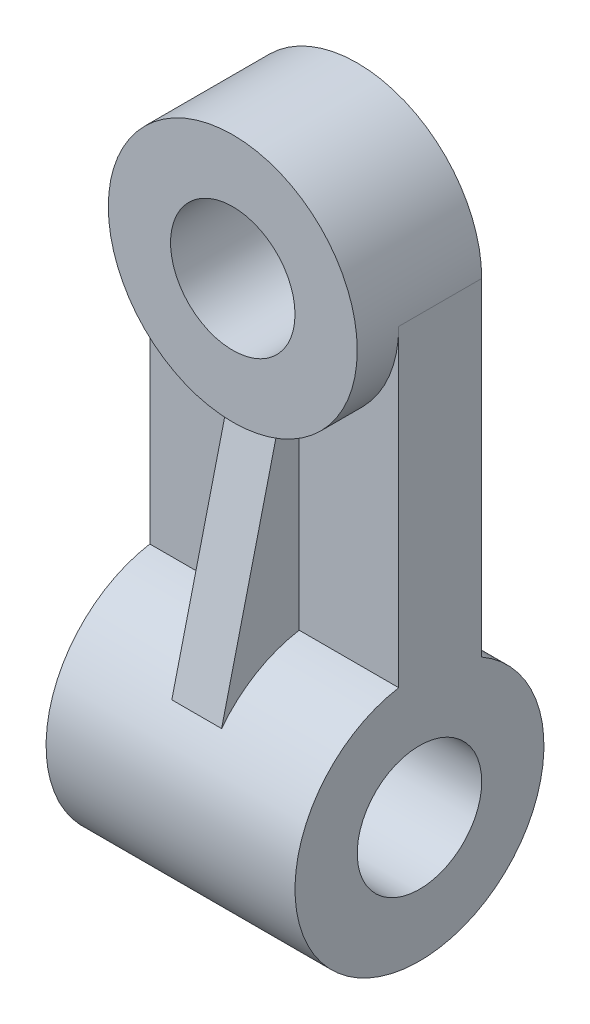
ISO-10303-21;
HEADER;
FILE_DESCRIPTION(('STEP AP214'),'2;1');
FILE_NAME('part.step','',(''),(''),'','','');
FILE_SCHEMA(('AUTOMOTIVE_DESIGN { 1 0 10303 214 1 1 1 1 }'));
ENDSEC;
DATA;
#1=APPLICATION_CONTEXT('core data for automotive mechanical design processes');
#2=APPLICATION_PROTOCOL_DEFINITION('international standard','automotive_design',2000,#1);
#3=PRODUCT_CONTEXT('',#1,'mechanical');
#4=PRODUCT('Part','Part','',(#3));
#5=PRODUCT_RELATED_PRODUCT_CATEGORY('part','',(#4));
#6=PRODUCT_DEFINITION_FORMATION('','',#4);
#7=PRODUCT_DEFINITION_CONTEXT('part definition',#1,'design');
#8=PRODUCT_DEFINITION('design','',#6,#7);
#9=PRODUCT_DEFINITION_SHAPE('','',#8);
#10=(LENGTH_UNIT() NAMED_UNIT(*) SI_UNIT(.MILLI.,.METRE.));
#11=(NAMED_UNIT(*) PLANE_ANGLE_UNIT() SI_UNIT($,.RADIAN.));
#12=(NAMED_UNIT(*) SI_UNIT($,.STERADIAN.) SOLID_ANGLE_UNIT());
#13=UNCERTAINTY_MEASURE_WITH_UNIT(LENGTH_MEASURE(1.E-05),#10,'distance_accuracy_value','');
#14=(GEOMETRIC_REPRESENTATION_CONTEXT(3) GLOBAL_UNCERTAINTY_ASSIGNED_CONTEXT((#13)) GLOBAL_UNIT_ASSIGNED_CONTEXT((#10,
#11,#12)) REPRESENTATION_CONTEXT('',''));
#15=CARTESIAN_POINT('',(0.,0.,0.));
#16=DIRECTION('',(0.,0.,1.));
#17=DIRECTION('',(1.,0.,0.));
#18=AXIS2_PLACEMENT_3D('',#15,#16,#17);
#19=CARTESIAN_POINT('',(30.,0.,20.));
#20=DIRECTION('',(0.,0.,-1.));
#21=DIRECTION('',(-1.,0.,0.));
#22=AXIS2_PLACEMENT_3D('',#19,#20,#21);
#23=PLANE('',#22);
#24=DIRECTION('',(0.,-1.,0.));
#25=VECTOR('',#24,1.);
#26=CARTESIAN_POINT('',(-6.,0.,20.));
#27=LINE('',#26,#25);
#28=CARTESIAN_POINT('',(-6.,-29.3938769133981,20.));
#29=VERTEX_POINT('',#28);
#30=CARTESIAN_POINT('',(-5.99999999999999,-75.4196010845019,20.));
#31=VERTEX_POINT('',#30);
#32=EDGE_CURVE('E116',#29,#31,#27,.T.);
#33=ORIENTED_EDGE('',*,*,#32,.F.);
#34=CARTESIAN_POINT('',(0.,0.,20.));
#35=DIRECTION('',(0.,0.,-1.));
#36=DIRECTION('',(-1.,0.,0.));
#37=AXIS2_PLACEMENT_3D('',#34,#35,#36);
#38=CIRCLE('',#37,30.);
#39=CARTESIAN_POINT('',(-30.,0.,20.));
#40=VERTEX_POINT('',#39);
#41=EDGE_CURVE('E160',#29,#40,#38,.T.);
#42=ORIENTED_EDGE('',*,*,#41,.T.);
#43=DIRECTION('',(0.,-1.,0.));
#44=VECTOR('',#43,1.);
#45=CARTESIAN_POINT('',(-30.,0.,20.));
#46=LINE('',#45,#44);
#47=CARTESIAN_POINT('',(-30.,-75.4196010845019,20.));
#48=VERTEX_POINT('',#47);
#49=EDGE_CURVE('E159',#40,#48,#46,.T.);
#50=ORIENTED_EDGE('',*,*,#49,.T.);
#51=DIRECTION('',(-1.,0.,0.));
#52=VECTOR('',#51,1.);
#53=CARTESIAN_POINT('',(30.,-75.4196010845019,20.));
#54=LINE('',#53,#52);
#55=EDGE_CURVE('E139',#31,#48,#54,.T.);
#56=ORIENTED_EDGE('',*,*,#55,.F.);
#57=EDGE_LOOP('',(#33,#42,#50,#56));
#58=FACE_BOUND('',#57,.T.);
#59=ADVANCED_FACE('F39',(#58),#23,.F.);
#60=CARTESIAN_POINT('',(0.,0.,0.));
#61=DIRECTION('',(0.,0.,1.));
#62=DIRECTION('',(1.,0.,0.));
#63=AXIS2_PLACEMENT_3D('',#60,#61,#62);
#64=PLANE('',#63);
#65=CARTESIAN_POINT('',(0.,0.,0.));
#66=DIRECTION('',(0.,0.,1.));
#67=DIRECTION('',(1.,0.,0.));
#68=AXIS2_PLACEMENT_3D('',#65,#66,#67);
#69=CIRCLE('',#68,15.);
#70=CARTESIAN_POINT('',(15.,0.,0.));
#71=VERTEX_POINT('',#70);
#72=EDGE_CURVE('E169',#71,#71,#69,.T.);
#73=ORIENTED_EDGE('',*,*,#72,.T.);
#74=EDGE_LOOP('',(#73));
#75=FACE_BOUND('',#74,.T.);
#76=DIRECTION('',(0.,1.,0.));
#77=VECTOR('',#76,1.);
#78=CARTESIAN_POINT('',(30.,-80.,0.));
#79=LINE('',#78,#77);
#80=CARTESIAN_POINT('',(30.,-79.0192378864668,0.));
#81=VERTEX_POINT('',#80);
#82=CARTESIAN_POINT('',(30.,0.,0.));
#83=VERTEX_POINT('',#82);
#84=EDGE_CURVE('E152',#81,#83,#79,.T.);
#85=ORIENTED_EDGE('',*,*,#84,.F.);
#86=DIRECTION('',(-1.,0.,0.));
#87=VECTOR('',#86,1.);
#88=CARTESIAN_POINT('',(30.,-79.0192378864668,0.));
#89=LINE('',#88,#87);
#90=CARTESIAN_POINT('',(-30.,-79.0192378864668,0.));
#91=VERTEX_POINT('',#90);
#92=EDGE_CURVE('E143',#91,#81,#89,.F.);
#93=ORIENTED_EDGE('',*,*,#92,.F.);
#94=DIRECTION('',(0.,1.,0.));
#95=VECTOR('',#94,1.);
#96=CARTESIAN_POINT('',(-30.,-80.,0.));
#97=LINE('',#96,#95);
#98=CARTESIAN_POINT('',(-30.,0.,0.));
#99=VERTEX_POINT('',#98);
#100=EDGE_CURVE('E151',#91,#99,#97,.T.);
#101=ORIENTED_EDGE('',*,*,#100,.T.);
#102=CARTESIAN_POINT('',(0.,0.,0.));
#103=DIRECTION('',(0.,0.,1.));
#104=DIRECTION('',(1.,0.,0.));
#105=AXIS2_PLACEMENT_3D('',#102,#103,#104);
#106=CIRCLE('',#105,30.);
#107=EDGE_CURVE('E175',#83,#99,#106,.T.);
#108=ORIENTED_EDGE('',*,*,#107,.F.);
#109=EDGE_LOOP('',(#85,#93,#101,#108));
#110=FACE_BOUND('',#109,.T.);
#111=ADVANCED_FACE('F183',(#75,#110),#64,.F.);
#112=CARTESIAN_POINT('',(30.,0.,20.));
#113=VERTEX_POINT('',#112);
#114=CARTESIAN_POINT('',(6.,-29.3938769133981,20.));
#115=VERTEX_POINT('',#114);
#116=EDGE_CURVE('E164',#113,#115,#38,.T.);
#117=ORIENTED_EDGE('',*,*,#116,.T.);
#118=DIRECTION('',(0.,-1.,0.));
#119=VECTOR('',#118,1.);
#120=CARTESIAN_POINT('',(6.,0.,20.));
#121=LINE('',#120,#119);
#122=CARTESIAN_POINT('',(6.00000000000001,-75.4196010845019,20.));
#123=VERTEX_POINT('',#122);
#124=EDGE_CURVE('E134',#115,#123,#121,.T.);
#125=ORIENTED_EDGE('',*,*,#124,.T.);
#126=CARTESIAN_POINT('',(30.,-75.4196010845019,20.));
#127=VERTEX_POINT('',#126);
#128=EDGE_CURVE('E141',#127,#123,#54,.T.);
#129=ORIENTED_EDGE('',*,*,#128,.F.);
#130=DIRECTION('',(0.,-1.,0.));
#131=VECTOR('',#130,1.);
#132=CARTESIAN_POINT('',(30.,0.,20.));
#133=LINE('',#132,#131);
#134=EDGE_CURVE('E154',#113,#127,#133,.T.);
#135=ORIENTED_EDGE('',*,*,#134,.F.);
#136=EDGE_LOOP('',(#117,#125,#129,#135));
#137=FACE_BOUND('',#136,.T.);
#138=ADVANCED_FACE('F191',(#137),#23,.F.);
#139=CARTESIAN_POINT('',(0.,0.,30.));
#140=DIRECTION('',(0.,0.,-1.));
#141=DIRECTION('',(-1.,0.,0.));
#142=AXIS2_PLACEMENT_3D('',#139,#140,#141);
#143=CYLINDRICAL_SURFACE('',#142,30.);
#144=CARTESIAN_POINT('',(0.,0.,30.));
#145=DIRECTION('',(0.,0.,1.));
#146=DIRECTION('',(1.,0.,0.));
#147=AXIS2_PLACEMENT_3D('',#144,#145,#146);
#148=CIRCLE('',#147,30.);
#149=CARTESIAN_POINT('',(30.,0.,30.));
#150=VERTEX_POINT('',#149);
#151=EDGE_CURVE('E120',#150,#150,#148,.T.);
#152=ORIENTED_EDGE('',*,*,#151,.F.);
#153=EDGE_LOOP('',(#152));
#154=FACE_BOUND('',#153,.T.);
#155=CARTESIAN_POINT('',(0.,0.,17.7414326109079));
#156=DIRECTION('',(0.,0.235166707699098,0.971955050190063));
#157=DIRECTION('',(0.,0.971955050190063,-0.235166707699098));
#158=AXIS2_PLACEMENT_3D('',#155,#156,#157);
#159=ELLIPSE('',#158,30.8656249012067,30.);
#160=CARTESIAN_POINT('',(-6.,-29.3938769133981,24.8533471576605));
#161=VERTEX_POINT('',#160);
#162=CARTESIAN_POINT('',(6.,-29.3938769133981,24.8533471576605));
#163=VERTEX_POINT('',#162);
#164=EDGE_CURVE('E53',#161,#163,#159,.T.);
#165=ORIENTED_EDGE('',*,*,#164,.T.);
#166=DIRECTION('',(0.,0.,-1.));
#167=VECTOR('',#166,1.);
#168=CARTESIAN_POINT('',(6.,-29.3938769133981,30.));
#169=LINE('',#168,#167);
#170=EDGE_CURVE('E135',#163,#115,#169,.T.);
#171=ORIENTED_EDGE('',*,*,#170,.T.);
#172=ORIENTED_EDGE('',*,*,#116,.F.);
#173=DIRECTION('',(0.,0.,1.));
#174=VECTOR('',#173,1.);
#175=CARTESIAN_POINT('',(30.,0.,0.));
#176=LINE('',#175,#174);
#177=EDGE_CURVE('E149',#83,#113,#176,.T.);
#178=ORIENTED_EDGE('',*,*,#177,.F.);
#179=ORIENTED_EDGE('',*,*,#107,.T.);
#180=DIRECTION('',(0.,0.,1.));
#181=VECTOR('',#180,1.);
#182=CARTESIAN_POINT('',(-30.,0.,0.));
#183=LINE('',#182,#181);
#184=EDGE_CURVE('E150',#99,#40,#183,.T.);
#185=ORIENTED_EDGE('',*,*,#184,.T.);
#186=ORIENTED_EDGE('',*,*,#41,.F.);
#187=DIRECTION('',(0.,0.,-1.));
#188=VECTOR('',#187,1.);
#189=CARTESIAN_POINT('',(-6.,-29.3938769133981,30.));
#190=LINE('',#189,#188);
#191=EDGE_CURVE('E56',#161,#29,#190,.T.);
#192=ORIENTED_EDGE('',*,*,#191,.F.);
#193=EDGE_LOOP('',(#165,#171,#172,#178,#179,#185,#186,#192));
#194=FACE_BOUND('',#193,.T.);
#195=ADVANCED_FACE('F41',(#154,#194),#143,.T.);
#196=CARTESIAN_POINT('',(0.,0.,0.));
#197=DIRECTION('',(0.,0.,1.));
#198=DIRECTION('',(1.,0.,0.));
#199=AXIS2_PLACEMENT_3D('',#196,#197,#198);
#200=CYLINDRICAL_SURFACE('',#199,15.);
#201=ORIENTED_EDGE('',*,*,#72,.F.);
#202=EDGE_LOOP('',(#201));
#203=FACE_BOUND('',#202,.T.);
#204=CARTESIAN_POINT('',(0.,0.,30.));
#205=DIRECTION('',(0.,0.,1.));
#206=DIRECTION('',(1.,0.,0.));
#207=AXIS2_PLACEMENT_3D('',#204,#205,#206);
#208=CIRCLE('',#207,15.);
#209=CARTESIAN_POINT('',(15.,0.,30.));
#210=VERTEX_POINT('',#209);
#211=EDGE_CURVE('E166',#210,#210,#208,.T.);
#212=ORIENTED_EDGE('',*,*,#211,.T.);
#213=EDGE_LOOP('',(#212));
#214=FACE_BOUND('',#213,.T.);
#215=ADVANCED_FACE('F223',(#203,#214),#200,.F.);
#216=CARTESIAN_POINT('',(0.,0.,30.));
#217=DIRECTION('',(0.,0.,1.));
#218=DIRECTION('',(1.,0.,0.));
#219=AXIS2_PLACEMENT_3D('',#216,#217,#218);
#220=PLANE('',#219);
#221=ORIENTED_EDGE('',*,*,#211,.F.);
#222=EDGE_LOOP('',(#221));
#223=FACE_BOUND('',#222,.T.);
#224=ORIENTED_EDGE('',*,*,#151,.T.);
#225=EDGE_LOOP('',(#224));
#226=FACE_BOUND('',#225,.T.);
#227=ADVANCED_FACE('F228',(#223,#226),#220,.T.);
#228=CARTESIAN_POINT('',(30.,0.,0.));
#229=DIRECTION('',(1.,0.,0.));
#230=DIRECTION('',(0.,0.,-1.));
#231=AXIS2_PLACEMENT_3D('',#228,#229,#230);
#232=PLANE('',#231);
#233=CARTESIAN_POINT('',(30.,-105.,15.));
#234=DIRECTION('',(1.,0.,0.));
#235=DIRECTION('',(0.,0.,-1.));
#236=AXIS2_PLACEMENT_3D('',#233,#234,#235);
#237=CIRCLE('',#236,15.);
#238=CARTESIAN_POINT('',(30.,-105.,0.));
#239=VERTEX_POINT('',#238);
#240=EDGE_CURVE('E123',#239,#239,#237,.T.);
#241=ORIENTED_EDGE('',*,*,#240,.F.);
#242=EDGE_LOOP('',(#241));
#243=FACE_BOUND('',#242,.T.);
#244=CARTESIAN_POINT('',(30.,-105.,15.));
#245=DIRECTION('',(1.,0.,0.));
#246=DIRECTION('',(0.,0.,-1.));
#247=AXIS2_PLACEMENT_3D('',#244,#245,#246);
#248=CIRCLE('',#247,30.);
#249=EDGE_CURVE('E140',#127,#81,#248,.T.);
#250=ORIENTED_EDGE('',*,*,#249,.T.);
#251=ORIENTED_EDGE('',*,*,#84,.T.);
#252=ORIENTED_EDGE('',*,*,#177,.T.);
#253=ORIENTED_EDGE('',*,*,#134,.T.);
#254=EDGE_LOOP('',(#250,#251,#252,#253));
#255=FACE_BOUND('',#254,.T.);
#256=ADVANCED_FACE('F192',(#243,#255),#232,.T.);
#257=CARTESIAN_POINT('',(-30.,0.,0.));
#258=DIRECTION('',(1.,0.,0.));
#259=DIRECTION('',(0.,0.,-1.));
#260=AXIS2_PLACEMENT_3D('',#257,#258,#259);
#261=PLANE('',#260);
#262=CARTESIAN_POINT('',(-30.,-105.,15.));
#263=DIRECTION('',(1.,0.,0.));
#264=DIRECTION('',(0.,0.,-1.));
#265=AXIS2_PLACEMENT_3D('',#262,#263,#264);
#266=CIRCLE('',#265,15.);
#267=CARTESIAN_POINT('',(-30.,-105.,0.));
#268=VERTEX_POINT('',#267);
#269=EDGE_CURVE('E122',#268,#268,#266,.T.);
#270=ORIENTED_EDGE('',*,*,#269,.T.);
#271=EDGE_LOOP('',(#270));
#272=FACE_BOUND('',#271,.T.);
#273=ORIENTED_EDGE('',*,*,#100,.F.);
#274=CARTESIAN_POINT('',(-30.,-105.,15.));
#275=DIRECTION('',(1.,0.,0.));
#276=DIRECTION('',(0.,0.,-1.));
#277=AXIS2_PLACEMENT_3D('',#274,#275,#276);
#278=CIRCLE('',#277,30.);
#279=EDGE_CURVE('E138',#48,#91,#278,.T.);
#280=ORIENTED_EDGE('',*,*,#279,.F.);
#281=ORIENTED_EDGE('',*,*,#49,.F.);
#282=ORIENTED_EDGE('',*,*,#184,.F.);
#283=EDGE_LOOP('',(#273,#280,#281,#282));
#284=FACE_BOUND('',#283,.T.);
#285=ADVANCED_FACE('F190',(#272,#284),#261,.F.);
#286=CARTESIAN_POINT('',(30.,-105.,15.));
#287=DIRECTION('',(-1.,0.,0.));
#288=DIRECTION('',(0.,0.,1.));
#289=AXIS2_PLACEMENT_3D('',#286,#287,#288);
#290=CYLINDRICAL_SURFACE('',#289,30.);
#291=ORIENTED_EDGE('',*,*,#92,.T.);
#292=ORIENTED_EDGE('',*,*,#249,.F.);
#293=ORIENTED_EDGE('',*,*,#128,.T.);
#294=CARTESIAN_POINT('',(6.,-105.,15.));
#295=DIRECTION('',(1.,0.,0.));
#296=DIRECTION('',(0.,0.,-1.));
#297=AXIS2_PLACEMENT_3D('',#294,#295,#296);
#298=CIRCLE('',#297,30.);
#299=CARTESIAN_POINT('',(6.,-86.5995734980517,38.6943939476493));
#300=VERTEX_POINT('',#299);
#301=EDGE_CURVE('E11',#123,#300,#298,.T.);
#302=ORIENTED_EDGE('',*,*,#301,.T.);
#303=DIRECTION('',(-1.,0.,0.));
#304=VECTOR('',#303,1.);
#305=CARTESIAN_POINT('',(30.,-86.5995734980517,38.6943939476493));
#306=LINE('',#305,#304);
#307=CARTESIAN_POINT('',(-6.,-86.5995734980517,38.6943939476493));
#308=VERTEX_POINT('',#307);
#309=EDGE_CURVE('E50',#300,#308,#306,.T.);
#310=ORIENTED_EDGE('',*,*,#309,.T.);
#311=CARTESIAN_POINT('',(-6.,-105.,15.));
#312=DIRECTION('',(1.,0.,0.));
#313=DIRECTION('',(0.,0.,-1.));
#314=AXIS2_PLACEMENT_3D('',#311,#312,#313);
#315=CIRCLE('',#314,30.);
#316=EDGE_CURVE('E101',#31,#308,#315,.T.);
#317=ORIENTED_EDGE('',*,*,#316,.F.);
#318=ORIENTED_EDGE('',*,*,#55,.T.);
#319=ORIENTED_EDGE('',*,*,#279,.T.);
#320=EDGE_LOOP('',(#291,#292,#293,#302,#310,#317,#318,#319));
#321=FACE_BOUND('',#320,.T.);
#322=ADVANCED_FACE('F105',(#321),#290,.T.);
#323=CARTESIAN_POINT('',(0.,-30.,25.));
#324=DIRECTION('',(0.,0.235166707699098,0.971955050190063));
#325=DIRECTION('',(0.,-0.971955050190063,0.235166707699098));
#326=AXIS2_PLACEMENT_3D('',#323,#324,#325);
#327=PLANE('',#326);
#328=ORIENTED_EDGE('',*,*,#164,.F.);
#329=DIRECTION('',(0.,-0.971955050190063,0.235166707699098));
#330=VECTOR('',#329,1.);
#331=CARTESIAN_POINT('',(-6.,-30.,25.));
#332=LINE('',#331,#330);
#333=EDGE_CURVE('E114',#161,#308,#332,.T.);
#334=ORIENTED_EDGE('',*,*,#333,.T.);
#335=ORIENTED_EDGE('',*,*,#309,.F.);
#336=DIRECTION('',(0.,-0.971955050190063,0.235166707699098));
#337=VECTOR('',#336,1.);
#338=CARTESIAN_POINT('',(6.,-30.,25.));
#339=LINE('',#338,#337);
#340=EDGE_CURVE('E119',#163,#300,#339,.T.);
#341=ORIENTED_EDGE('',*,*,#340,.F.);
#342=EDGE_LOOP('',(#328,#334,#335,#341));
#343=FACE_BOUND('',#342,.T.);
#344=ADVANCED_FACE('F118',(#343),#327,.T.);
#345=CARTESIAN_POINT('',(6.,-52.5,15.));
#346=DIRECTION('',(1.,0.,0.));
#347=DIRECTION('',(0.,0.,-1.));
#348=AXIS2_PLACEMENT_3D('',#345,#346,#347);
#349=PLANE('',#348);
#350=ORIENTED_EDGE('',*,*,#170,.F.);
#351=ORIENTED_EDGE('',*,*,#340,.T.);
#352=ORIENTED_EDGE('',*,*,#301,.F.);
#353=ORIENTED_EDGE('',*,*,#124,.F.);
#354=EDGE_LOOP('',(#350,#351,#352,#353));
#355=FACE_BOUND('',#354,.T.);
#356=ADVANCED_FACE('F196',(#355),#349,.T.);
#357=CARTESIAN_POINT('',(-6.,-52.5,15.));
#358=DIRECTION('',(1.,0.,0.));
#359=DIRECTION('',(0.,0.,-1.));
#360=AXIS2_PLACEMENT_3D('',#357,#358,#359);
#361=PLANE('',#360);
#362=ORIENTED_EDGE('',*,*,#333,.F.);
#363=ORIENTED_EDGE('',*,*,#191,.T.);
#364=ORIENTED_EDGE('',*,*,#32,.T.);
#365=ORIENTED_EDGE('',*,*,#316,.T.);
#366=EDGE_LOOP('',(#362,#363,#364,#365));
#367=FACE_BOUND('',#366,.T.);
#368=ADVANCED_FACE('F112',(#367),#361,.F.);
#369=CARTESIAN_POINT('',(-30.,-105.,15.));
#370=DIRECTION('',(1.,0.,0.));
#371=DIRECTION('',(0.,0.,-1.));
#372=AXIS2_PLACEMENT_3D('',#369,#370,#371);
#373=CYLINDRICAL_SURFACE('',#372,15.);
#374=CARTESIAN_POINT('',(-30.,-105.,0.));
#375=CARTESIAN_POINT('',(-29.375,-105.,0.));
#376=CARTESIAN_POINT('',(-28.75,-105.,0.));
#377=CARTESIAN_POINT('',(-27.5,-105.,0.));
#378=CARTESIAN_POINT('',(-26.875,-105.,0.));
#379=CARTESIAN_POINT('',(-25.625,-105.,0.));
#380=CARTESIAN_POINT('',(-25.,-105.,0.));
#381=CARTESIAN_POINT('',(-23.75,-105.,0.));
#382=CARTESIAN_POINT('',(-23.125,-105.,0.));
#383=CARTESIAN_POINT('',(-21.875,-105.,0.));
#384=CARTESIAN_POINT('',(-21.25,-105.,0.));
#385=CARTESIAN_POINT('',(-20.,-105.,0.));
#386=CARTESIAN_POINT('',(-19.375,-105.,0.));
#387=CARTESIAN_POINT('',(-18.125,-105.,0.));
#388=CARTESIAN_POINT('',(-17.5,-105.,0.));
#389=CARTESIAN_POINT('',(-16.25,-105.,0.));
#390=CARTESIAN_POINT('',(-15.625,-105.,0.));
#391=CARTESIAN_POINT('',(-14.375,-105.,0.));
#392=CARTESIAN_POINT('',(-13.75,-105.,0.));
#393=CARTESIAN_POINT('',(-12.5,-105.,0.));
#394=CARTESIAN_POINT('',(-11.875,-105.,0.));
#395=CARTESIAN_POINT('',(-10.625,-105.,0.));
#396=CARTESIAN_POINT('',(-10.,-105.,0.));
#397=CARTESIAN_POINT('',(-8.75,-105.,0.));
#398=CARTESIAN_POINT('',(-8.125,-105.,0.));
#399=CARTESIAN_POINT('',(-6.875,-105.,0.));
#400=CARTESIAN_POINT('',(-6.25,-105.,0.));
#401=CARTESIAN_POINT('',(-5.,-105.,0.));
#402=CARTESIAN_POINT('',(-4.375,-105.,0.));
#403=CARTESIAN_POINT('',(-3.125,-105.,0.));
#404=CARTESIAN_POINT('',(-2.5,-105.,0.));
#405=CARTESIAN_POINT('',(-1.25,-105.,0.));
#406=CARTESIAN_POINT('',(-0.625,-105.,0.));
#407=CARTESIAN_POINT('',(0.624999999999999,-105.,0.));
#408=CARTESIAN_POINT('',(1.25,-105.,0.));
#409=CARTESIAN_POINT('',(2.5,-105.,0.));
#410=CARTESIAN_POINT('',(3.125,-105.,0.));
#411=CARTESIAN_POINT('',(4.375,-105.,0.));
#412=CARTESIAN_POINT('',(5.,-105.,0.));
#413=CARTESIAN_POINT('',(6.25,-105.,0.));
#414=CARTESIAN_POINT('',(6.875,-105.,0.));
#415=CARTESIAN_POINT('',(8.125,-105.,0.));
#416=CARTESIAN_POINT('',(8.75,-105.,0.));
#417=CARTESIAN_POINT('',(10.,-105.,0.));
#418=CARTESIAN_POINT('',(10.625,-105.,0.));
#419=CARTESIAN_POINT('',(11.875,-105.,0.));
#420=CARTESIAN_POINT('',(12.5,-105.,0.));
#421=CARTESIAN_POINT('',(13.75,-105.,0.));
#422=CARTESIAN_POINT('',(14.375,-105.,0.));
#423=CARTESIAN_POINT('',(15.625,-105.,0.));
#424=CARTESIAN_POINT('',(16.25,-105.,0.));
#425=CARTESIAN_POINT('',(17.5,-105.,0.));
#426=CARTESIAN_POINT('',(18.125,-105.,0.));
#427=CARTESIAN_POINT('',(19.375,-105.,0.));
#428=CARTESIAN_POINT('',(20.,-105.,0.));
#429=CARTESIAN_POINT('',(21.25,-105.,0.));
#430=CARTESIAN_POINT('',(21.875,-105.,0.));
#431=CARTESIAN_POINT('',(23.125,-105.,0.));
#432=CARTESIAN_POINT('',(23.75,-105.,0.));
#433=CARTESIAN_POINT('',(25.,-105.,0.));
#434=CARTESIAN_POINT('',(25.625,-105.,0.));
#435=CARTESIAN_POINT('',(26.875,-105.,0.));
#436=CARTESIAN_POINT('',(27.5,-105.,0.));
#437=CARTESIAN_POINT('',(28.75,-105.,0.));
#438=CARTESIAN_POINT('',(29.375,-105.,0.));
#439=CARTESIAN_POINT('',(30.,-105.,0.));
#440=B_SPLINE_CURVE_WITH_KNOTS('',3,(#374,#375,#376,#377,#378,#379,#380,#381,#382,#383,#384,
#385,#386,#387,#388,#389,#390,#391,#392,#393,#394,#395,#396,#397,#398,#399,#400,#401,#402,#403,
#404,#405,#406,#407,#408,#409,#410,#411,#412,#413,#414,#415,#416,#417,#418,#419,#420,#421,#422,
#423,#424,#425,#426,#427,#428,#429,#430,#431,#432,#433,#434,#435,#436,#437,#438,#439),
.UNSPECIFIED.,.F.,.F.,(4,2,2,2,2,2,2,2,2,2,2,2,2,2,2,2,2,2,2,2,2,2,2,2,2,2,2,2,2,2,2,2,4),(0.,
1.875,3.75,5.625,7.5,9.375,11.25,13.125,15.,16.875,18.75,20.625,22.5,24.375,26.25,28.125,30.,
31.875,33.75,35.625,37.5,39.375,41.25,43.125,45.,46.875,48.75,50.625,52.5,54.375,56.25,58.125,
60.),.UNSPECIFIED.);
#441=EDGE_CURVE('BSEAM202',#268,#239,#440,.T.);
#442=ORIENTED_EDGE('',*,*,#269,.F.);
#443=ORIENTED_EDGE('',*,*,#240,.T.);
#444=ORIENTED_EDGE('',*,*,#441,.T.);
#445=ORIENTED_EDGE('',*,*,#441,.F.);
#446=EDGE_LOOP('',(#442,#444,#443,#445));
#447=FACE_BOUND('',#446,.T.);
#448=ADVANCED_FACE('F202',(#447),#373,.F.);
#449=CLOSED_SHELL('',(#59,#111,#138,#195,#215,#227,#256,#285,#322,#344,#356,#368,#448));
#450=MANIFOLD_SOLID_BREP('B2',#449);
#451=ADVANCED_BREP_SHAPE_REPRESENTATION('',(#18,#450),#14);
#452=SHAPE_DEFINITION_REPRESENTATION(#9,#451);
ENDSEC;
END-ISO-10303-21;
